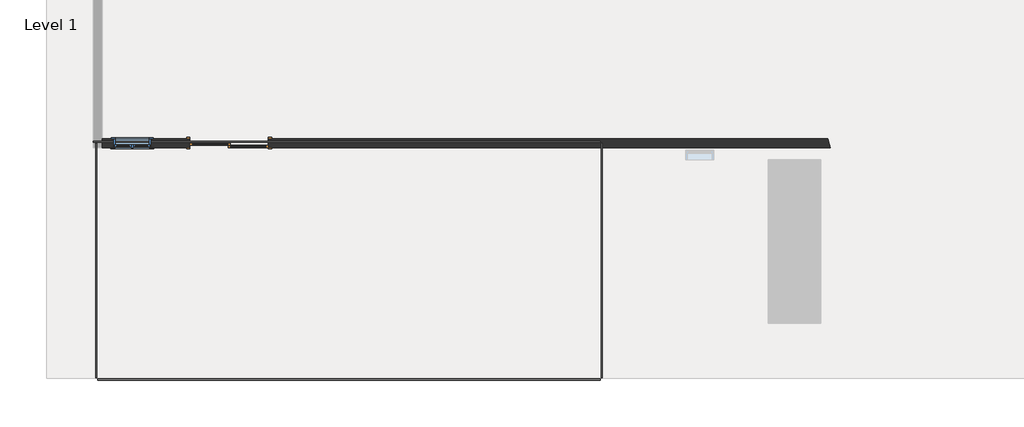
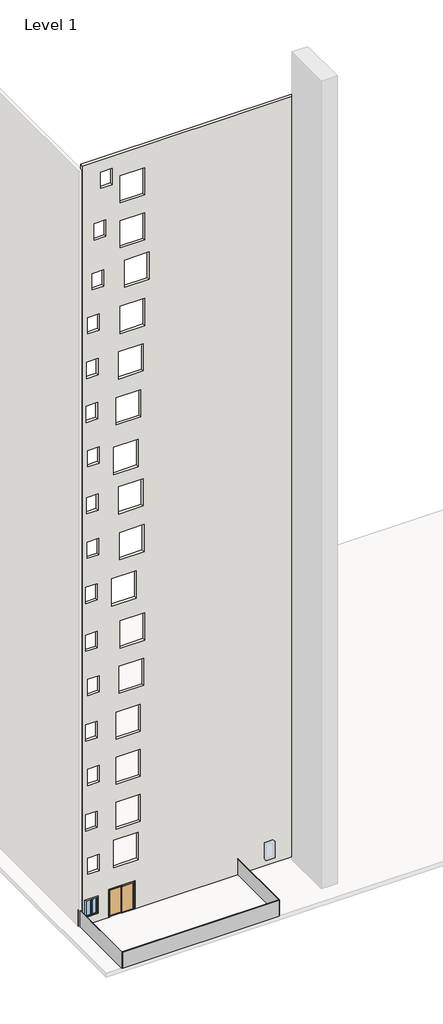
# One storey, part 1 of 3: 4 plates, 1 door, 1 wall, 1 window.
"""IFC4 building model written with IfcOpenShell, lengths in millimetres."""

from ifc_helpers import new_model, si_unit, frame, origin, place, context, project, spatial, polyline, circle_curve, transform, mapped, element, save
from ifc_brep_helpers import plane_surface, revolved_surface, advanced_brep
from components import door_076b30e0, system_panel_glazed_d9738348, system_panel_glazed_605ab5bb, system_panel_glazed_d159b752, window_bb17773d

model = new_model("IFC4")

# Units and contexts
model_context = context("Model", 3, world=origin())
ifc_project = project(units=[si_unit("LENGTHUNIT", "METRE", prefix="MILLI")], contexts=[model_context])

# Site, building, storey
site = spatial("IfcSite", under=ifc_project)
building = spatial("IfcBuilding", under=site)
storey = spatial("IfcBuildingStorey", under=building, Name="Level 1", Elevation=0.0)

# Door
placement = place(None, origin())
door_shape = door_076b30e0(model_context)
element("IfcDoor", 1, ObjectType="Door-Double-Sliding : 68\" x 80\"", at=placement, inside=storey, context=model_context, shape_type="MappedRepresentation", body=[
    mapped(door_shape, transform((-16826.585279, -12227.7237084, 0.0), x_axis=(-1.0, 0.0, 0.0), y_axis=(0.0, -1.0, 0.0), z_axis=(0.0, 0.0, 1.0))),
])

# Plates
system_panel_glazed_shape = system_panel_glazed_d9738348(model_context)
element("IfcPlate", 2, ObjectType="System Panel : Glazed", at=placement, inside=storey, context=model_context, shape_type="MappedRepresentation", body=[
    mapped(system_panel_glazed_shape, transform((-14188.160279, -17528.1341134, 0.0), x_axis=(-1.0, 0.0, 0.0), y_axis=(0.0, -1.0, 0.0), z_axis=(0.0, 0.0, 1.0))),
])
system_panel_glazed_2_shape = system_panel_glazed_605ab5bb(model_context)
element("IfcPlate", 3, ObjectType="System Panel : Glazed", at=placement, inside=storey, context=model_context, shape_type="MappedRepresentation", body=[
    mapped(system_panel_glazed_2_shape, transform((-19722.185279, -14941.4289109, 0.0), x_axis=(0.0, 1.0, 0.0), y_axis=(-1.0, 0.0, 0.0), z_axis=(0.0, 0.0, 1.0))),
])
element("IfcPlate", 4, ObjectType="System Panel : Glazed", at=placement, inside=storey, context=model_context, shape_type="MappedRepresentation", body=[
    mapped(system_panel_glazed_2_shape, transform((-8654.135279, -14941.4289109, 0.0), x_axis=(0.0, -1.0, 0.0), y_axis=(1.0, 0.0, 0.0), z_axis=(0.0, 0.0, 1.0))),
])
system_panel_glazed_3_shape = system_panel_glazed_d159b752(model_context)
element("IfcPlate", 5, ObjectType="System Panel : Glazed", at=placement, inside=storey, context=model_context, shape_type="MappedRepresentation", body=[
    mapped(system_panel_glazed_3_shape, transform((-14238.960279, -12354.7237084, 0.0), x_axis=(1.0, 0.0, 0.0), y_axis=(0.0, 1.0, 0.0), z_axis=(0.0, 0.0, 1.0))),
])

# Wall
element("IfcWall", 6, ObjectType="Generic - 8\"", at=placement, inside=storey, context=model_context, shape_type="AdvancedBrep", body=[
    advanced_brep(
    [(-17690.185279, -12253.1237084, 2032.0), (-17690.185279, -12253.1237084, 0.0), (-19620.585279, -12253.1237084, 0.0), (-19620.585279, -12253.1237084, 56730.1367162), (-3637.9363527, -12253.1237084, 56730.1367162), (-3637.9363527, -12253.1237084, 0.0), (-15962.985279, -12253.1237084, 0.0), (-15962.985279, -12253.1237084, 2032.0), (-18299.785279, -12253.1237084, 55822.814928), (-18299.785279, -12253.1237084, 54603.614928), (-17486.985279, -12253.1237084, 54603.614928), (-17486.985279, -12253.1237084, 55822.814928), (-18756.985279, -12253.1237084, 52120.8), (-18756.985279, -12253.1237084, 50901.6), (-17944.185279, -12253.1237084, 50901.6), (-17944.185279, -12253.1237084, 52120.8), (-18909.385279, -12253.1237084, 48463.2), (-18909.385279, -12253.1237084, 47244.0), (-18096.585279, -12253.1237084, 47244.0), (-18096.585279, -12253.1237084, 48463.2), (-19214.185279, -12253.1237084, 45287.1858782), (-19214.185279, -12253.1237084, 44067.9858782), (-18401.385279, -12253.1237084, 44067.9858782), (-18401.385279, -12253.1237084, 45287.1858782), (-19315.785279, -12253.1237084, 41987.2293246), (-19315.785279, -12253.1237084, 40768.0293246), (-18502.985279, -12253.1237084, 40768.0293246), (-18502.985279, -12253.1237084, 41987.2293246), (-19341.185279, -12253.1237084, 38709.6), (-19341.185279, -12253.1237084, 37490.4), (-18528.385279, -12253.1237084, 37490.4), (-18528.385279, -12253.1237084, 38709.6), (-19214.185279, -12253.1237084, 35356.8), (-19214.185279, -12253.1237084, 34137.6), (-18401.385279, -12253.1237084, 34137.6), (-18401.385279, -12253.1237084, 35356.8), (-19315.785279, -12253.1237084, 31888.4931655), (-19315.785279, -12253.1237084, 30669.2931655), (-18502.985279, -12253.1237084, 30669.2931655), (-18502.985279, -12253.1237084, 31888.4931655), (-19264.985279, -12253.1237084, 28544.0955009), (-19264.985279, -12253.1237084, 27324.8955009), (-18452.185279, -12253.1237084, 27324.8955009), (-18452.185279, -12253.1237084, 28544.0955009), (-19366.585279, -12253.1237084, 25208.6161382), (-19366.585279, -12253.1237084, 23989.4161382), (-18553.785279, -12253.1237084, 23989.4161382), (-18553.785279, -12253.1237084, 25208.6161382), (-19366.585279, -12253.1237084, 21640.8), (-19366.585279, -12253.1237084, 20421.6), (-18553.785279, -12253.1237084, 20421.6), (-18553.785279, -12253.1237084, 21640.8), (-19214.185279, -12253.1237084, 18288.0), (-19214.185279, -12253.1237084, 17068.8), (-18401.385279, -12253.1237084, 17068.8), (-18401.385279, -12253.1237084, 18288.0), (-19366.585279, -12253.1237084, 14935.2), (-19366.585279, -12253.1237084, 13716.0), (-18553.785279, -12253.1237084, 13716.0), (-18553.785279, -12253.1237084, 14935.2), (-19214.185279, -12253.1237084, 11582.4), (-19214.185279, -12253.1237084, 10363.2), (-18401.385279, -12253.1237084, 10363.2), (-18401.385279, -12253.1237084, 11582.4), (-19366.585279, -12253.1237084, 8229.6), (-19366.585279, -12253.1237084, 7010.4), (-18553.785279, -12253.1237084, 7010.4), (-18553.785279, -12253.1237084, 8229.6), (-19214.185279, -12253.1237084, 4949.2094119), (-19214.185279, -12253.1237084, 3730.0094119), (-18401.385279, -12253.1237084, 3730.0094119), (-18401.385279, -12253.1237084, 4949.2094119), (-19366.585279, -12253.1237084, 1819.2734472), (-19366.585279, -12253.1237084, 600.0734472), (-18553.785279, -12253.1237084, 600.0734472), (-18553.785279, -12253.1237084, 1819.2734472), (-15277.185279, -12253.1237084, 18491.2), (-17004.385279, -12253.1237084, 18491.2), (-17004.385279, -12253.1237084, 16459.2), (-15277.185279, -12253.1237084, 16459.2), (-15200.985279, -12253.1237084, 21844.0), (-16928.185279, -12253.1237084, 21844.0), (-16928.185279, -12253.1237084, 19812.0), (-15200.985279, -12253.1237084, 19812.0), (-15505.785279, -12253.1237084, 15138.4), (-17232.985279, -12253.1237084, 15138.4), (-17232.985279, -12253.1237084, 13106.4), (-15505.785279, -12253.1237084, 13106.4), (-15505.785279, -12253.1237084, 11785.6), (-17232.985279, -12253.1237084, 11785.6), (-17232.985279, -12253.1237084, 9753.6), (-15505.785279, -12253.1237084, 9753.6), (-15505.785279, -12253.1237084, 8432.8), (-17232.985279, -12253.1237084, 8432.8), (-17232.985279, -12253.1237084, 6400.8), (-15505.785279, -12253.1237084, 6400.8), (-15658.185279, -12253.1237084, 5624.1911771), (-17385.385279, -12253.1237084, 5624.1911771), (-17385.385279, -12253.1237084, 3592.1911771), (-15658.185279, -12253.1237084, 3592.1911771), (-15810.585279, -12253.1237084, 25196.8), (-17537.785279, -12253.1237084, 25196.8), (-17537.785279, -12253.1237084, 23164.8), (-15810.585279, -12253.1237084, 23164.8), (-15251.785279, -12253.1237084, 28462.5574534), (-16978.985279, -12253.1237084, 28462.5574534), (-16978.985279, -12253.1237084, 26430.5574534), (-15251.785279, -12253.1237084, 26430.5574534), (-15327.985279, -12253.1237084, 31902.4), (-17055.185279, -12253.1237084, 31902.4), (-17055.185279, -12253.1237084, 29870.4), (-15327.985279, -12253.1237084, 29870.4), (-15658.185279, -12253.1237084, 34950.4), (-17385.385279, -12253.1237084, 34950.4), (-17385.385279, -12253.1237084, 32918.4), (-15658.185279, -12253.1237084, 32918.4), (-15480.385279, -12253.1237084, 38608.0), (-17207.585279, -12253.1237084, 38608.0), (-17207.585279, -12253.1237084, 36576.0), (-15480.385279, -12253.1237084, 36576.0), (-15302.585279, -12253.1237084, 41960.8), (-17029.785279, -12253.1237084, 41960.8), (-17029.785279, -12253.1237084, 39928.8), (-15302.585279, -12253.1237084, 39928.8), (-15200.985279, -12253.1237084, 45313.6), (-16928.185279, -12253.1237084, 45313.6), (-16928.185279, -12253.1237084, 43281.6), (-15200.985279, -12253.1237084, 43281.6), (-14896.185279, -12253.1237084, 48666.4), (-16623.385279, -12253.1237084, 48666.4), (-16623.385279, -12253.1237084, 46634.4), (-14896.185279, -12253.1237084, 46634.4), (-15200.985279, -12253.1237084, 51714.4), (-16928.185279, -12253.1237084, 51714.4), (-16928.185279, -12253.1237084, 49682.4), (-15200.985279, -12253.1237084, 49682.4), (-15200.985279, -12253.1237084, 55067.2), (-16928.185279, -12253.1237084, 55067.2), (-16928.185279, -12253.1237084, 53035.2), (-15200.985279, -12253.1237084, 53035.2), (-19620.585279, -12456.3237084, 0.0), (-17690.185279, -12456.3237084, 0.0), (-17690.185279, -12456.3237084, 2032.0), (-15962.985279, -12456.3237084, 2032.0), (-15962.985279, -12456.3237084, 0.0), (-3801.1300045, -12456.3237084, 0.0), (-3592.0543777, -12456.3237084, 0.0), (-3592.0543777, -12456.3237084, 56730.1367162), (-3801.1300045, -12456.3237084, 56730.1367162), (-19620.585279, -12456.3237084, 56730.1367162), (-19620.585279, -12456.3237084, 56425.3367162), (-18299.785279, -12456.3237084, 55822.814928), (-17486.985279, -12456.3237084, 55822.814928), (-17486.985279, -12456.3237084, 54603.614928), (-18299.785279, -12456.3237084, 54603.614928), (-18756.985279, -12456.3237084, 52120.8), (-17944.185279, -12456.3237084, 52120.8), (-17944.185279, -12456.3237084, 50901.6), (-18756.985279, -12456.3237084, 50901.6), (-18909.385279, -12456.3237084, 48463.2), (-18096.585279, -12456.3237084, 48463.2), (-18096.585279, -12456.3237084, 47244.0), (-18909.385279, -12456.3237084, 47244.0), (-19214.185279, -12456.3237084, 45287.1858782), (-18401.385279, -12456.3237084, 45287.1858782), (-18401.385279, -12456.3237084, 44067.9858782), (-19214.185279, -12456.3237084, 44067.9858782), (-19315.785279, -12456.3237084, 41987.2293246), (-18502.985279, -12456.3237084, 41987.2293246), (-18502.985279, -12456.3237084, 40768.0293246), (-19315.785279, -12456.3237084, 40768.0293246), (-19341.185279, -12456.3237084, 38709.6), (-18528.385279, -12456.3237084, 38709.6), (-18528.385279, -12456.3237084, 37490.4), (-19341.185279, -12456.3237084, 37490.4), (-19214.185279, -12456.3237084, 35356.8), (-18401.385279, -12456.3237084, 35356.8), (-18401.385279, -12456.3237084, 34137.6), (-19214.185279, -12456.3237084, 34137.6), (-19315.785279, -12456.3237084, 31888.4931655), (-18502.985279, -12456.3237084, 31888.4931655), (-18502.985279, -12456.3237084, 30669.2931655), (-19315.785279, -12456.3237084, 30669.2931655), (-19264.985279, -12456.3237084, 28544.0955009), (-18452.185279, -12456.3237084, 28544.0955009), (-18452.185279, -12456.3237084, 27324.8955009), (-19264.985279, -12456.3237084, 27324.8955009), (-19366.585279, -12456.3237084, 25208.6161382), (-18553.785279, -12456.3237084, 25208.6161382), (-18553.785279, -12456.3237084, 23989.4161382), (-19366.585279, -12456.3237084, 23989.4161382), (-19366.585279, -12456.3237084, 21640.8), (-18553.785279, -12456.3237084, 21640.8), (-18553.785279, -12456.3237084, 20421.6), (-19366.585279, -12456.3237084, 20421.6), (-19214.185279, -12456.3237084, 18288.0), (-18401.385279, -12456.3237084, 18288.0), (-18401.385279, -12456.3237084, 17068.8), (-19214.185279, -12456.3237084, 17068.8), (-19366.585279, -12456.3237084, 14935.2), (-18553.785279, -12456.3237084, 14935.2), (-18553.785279, -12456.3237084, 13716.0), (-19366.585279, -12456.3237084, 13716.0), (-19214.185279, -12456.3237084, 11582.4), (-18401.385279, -12456.3237084, 11582.4), (-18401.385279, -12456.3237084, 10363.2), (-19214.185279, -12456.3237084, 10363.2), (-19366.585279, -12456.3237084, 8229.6), (-18553.785279, -12456.3237084, 8229.6), (-18553.785279, -12456.3237084, 7010.4), (-19366.585279, -12456.3237084, 7010.4), (-19214.185279, -12456.3237084, 4949.2094119), (-18401.385279, -12456.3237084, 4949.2094119), (-18401.385279, -12456.3237084, 3730.0094119), (-19214.185279, -12456.3237084, 3730.0094119), (-19366.585279, -12456.3237084, 1819.2734472), (-18553.785279, -12456.3237084, 1819.2734472), (-18553.785279, -12456.3237084, 600.0734472), (-19366.585279, -12456.3237084, 600.0734472), (-15277.185279, -12456.3237084, 18491.2), (-15277.185279, -12456.3237084, 16459.2), (-17004.385279, -12456.3237084, 16459.2), (-17004.385279, -12456.3237084, 18491.2), (-15200.985279, -12456.3237084, 21844.0), (-15200.985279, -12456.3237084, 19812.0), (-16928.185279, -12456.3237084, 19812.0), (-16928.185279, -12456.3237084, 21844.0), (-15505.785279, -12456.3237084, 15138.4), (-15505.785279, -12456.3237084, 13106.4), (-17232.985279, -12456.3237084, 13106.4), (-17232.985279, -12456.3237084, 15138.4), (-15505.785279, -12456.3237084, 11785.6), (-15505.785279, -12456.3237084, 9753.6), (-17232.985279, -12456.3237084, 9753.6), (-17232.985279, -12456.3237084, 11785.6), (-15505.785279, -12456.3237084, 8432.8), (-15505.785279, -12456.3237084, 6400.8), (-17232.985279, -12456.3237084, 6400.8), (-17232.985279, -12456.3237084, 8432.8), (-15658.185279, -12456.3237084, 5624.1911771), (-15658.185279, -12456.3237084, 3592.1911771), (-17385.385279, -12456.3237084, 3592.1911771), (-17385.385279, -12456.3237084, 5624.1911771), (-15810.585279, -12456.3237084, 25196.8), (-15810.585279, -12456.3237084, 23164.8), (-17537.785279, -12456.3237084, 23164.8), (-17537.785279, -12456.3237084, 25196.8), (-15251.785279, -12456.3237084, 28462.5574534), (-15251.785279, -12456.3237084, 26430.5574534), (-16978.985279, -12456.3237084, 26430.5574534), (-16978.985279, -12456.3237084, 28462.5574534), (-15327.985279, -12456.3237084, 31902.4), (-15327.985279, -12456.3237084, 29870.4), (-17055.185279, -12456.3237084, 29870.4), (-17055.185279, -12456.3237084, 31902.4), (-15658.185279, -12456.3237084, 34950.4), (-15658.185279, -12456.3237084, 32918.4), (-17385.385279, -12456.3237084, 32918.4), (-17385.385279, -12456.3237084, 34950.4), (-15480.385279, -12456.3237084, 38608.0), (-15480.385279, -12456.3237084, 36576.0), (-17207.585279, -12456.3237084, 36576.0), (-17207.585279, -12456.3237084, 38608.0), (-15302.585279, -12456.3237084, 41960.8), (-15302.585279, -12456.3237084, 39928.8), (-17029.785279, -12456.3237084, 39928.8), (-17029.785279, -12456.3237084, 41960.8), (-15200.985279, -12456.3237084, 45313.6), (-15200.985279, -12456.3237084, 43281.6), (-16928.185279, -12456.3237084, 43281.6), (-16928.185279, -12456.3237084, 45313.6), (-14896.185279, -12456.3237084, 48666.4), (-14896.185279, -12456.3237084, 46634.4), (-16623.385279, -12456.3237084, 46634.4), (-16623.385279, -12456.3237084, 48666.4), (-15200.985279, -12456.3237084, 51714.4), (-15200.985279, -12456.3237084, 49682.4), (-16928.185279, -12456.3237084, 49682.4), (-16928.185279, -12456.3237084, 51714.4), (-15200.985279, -12456.3237084, 55067.2), (-15200.985279, -12456.3237084, 53035.2), (-16928.185279, -12456.3237084, 53035.2), (-16928.185279, -12456.3237084, 55067.2)],
    [
        (0, 1),
        (1, 2),
        (2, 3),
        (3, 4),
        (4, 5),
        (5, 6),
        (6, 7),
        (7, 0),
        (8, 9),
        (9, 10),
        (10, 11),
        (11, 8),
        (12, 13),
        (13, 14),
        (14, 15),
        (15, 12),
        (16, 17),
        (17, 18),
        (18, 19),
        (19, 16),
        (20, 21),
        (21, 22),
        (22, 23),
        (23, 20),
        (24, 25),
        (25, 26),
        (26, 27),
        (27, 24),
        (28, 29),
        (29, 30),
        (30, 31),
        (31, 28),
        (32, 33),
        (33, 34),
        (34, 35),
        (35, 32),
        (36, 37),
        (37, 38),
        (38, 39),
        (39, 36),
        (40, 41),
        (41, 42),
        (42, 43),
        (43, 40),
        (44, 45),
        (45, 46),
        (46, 47),
        (47, 44),
        (48, 49),
        (49, 50),
        (50, 51),
        (51, 48),
        (52, 53),
        (53, 54),
        (54, 55),
        (55, 52),
        (56, 57),
        (57, 58),
        (58, 59),
        (59, 56),
        (60, 61),
        (61, 62),
        (62, 63),
        (63, 60),
        (64, 65),
        (65, 66),
        (66, 67),
        (67, 64),
        (68, 69),
        (69, 70),
        (70, 71),
        (71, 68),
        (72, 73),
        (73, 74),
        (74, 75),
        (75, 72),
        (76, 77),
        (77, 78),
        (78, 79),
        (79, 76),
        (80, 81),
        (81, 82),
        (82, 83),
        (83, 80),
        (84, 85),
        (85, 86),
        (86, 87),
        (87, 84),
        (88, 89),
        (89, 90),
        (90, 91),
        (91, 88),
        (92, 93),
        (93, 94),
        (94, 95),
        (95, 92),
        (96, 97),
        (97, 98),
        (98, 99),
        (99, 96),
        (100, 101),
        (101, 102),
        (102, 103),
        (103, 100),
        (104, 105),
        (105, 106),
        (106, 107),
        (107, 104),
        (108, 109),
        (109, 110),
        (110, 111),
        (111, 108),
        (112, 113),
        (113, 114),
        (114, 115),
        (115, 112),
        (116, 117),
        (117, 118),
        (118, 119),
        (119, 116),
        (120, 121),
        (121, 122),
        (122, 123),
        (123, 120),
        (124, 125),
        (125, 126),
        (126, 127),
        (127, 124),
        (128, 129),
        (129, 130),
        (130, 131),
        (131, 128),
        (132, 133),
        (133, 134),
        (134, 135),
        (135, 132),
        (136, 137),
        (137, 138),
        (138, 139),
        (139, 136),
        (140, 141),
        (141, 142),
        (142, 143),
        (143, 144),
        (144, 145),
        (145, 146),
        (146, 147),
        (147, 148),
        (148, 149),
        (149, 150),
        (150, 140),
        (151, 152),
        (152, 153),
        (153, 154),
        (154, 151),
        (155, 156),
        (156, 157),
        (157, 158),
        (158, 155),
        (159, 160),
        (160, 161),
        (161, 162),
        (162, 159),
        (163, 164),
        (164, 165),
        (165, 166),
        (166, 163),
        (167, 168),
        (168, 169),
        (169, 170),
        (170, 167),
        (171, 172),
        (172, 173),
        (173, 174),
        (174, 171),
        (175, 176),
        (176, 177),
        (177, 178),
        (178, 175),
        (179, 180),
        (180, 181),
        (181, 182),
        (182, 179),
        (183, 184),
        (184, 185),
        (185, 186),
        (186, 183),
        (187, 188),
        (188, 189),
        (189, 190),
        (190, 187),
        (191, 192),
        (192, 193),
        (193, 194),
        (194, 191),
        (195, 196),
        (196, 197),
        (197, 198),
        (198, 195),
        (199, 200),
        (200, 201),
        (201, 202),
        (202, 199),
        (203, 204),
        (204, 205),
        (205, 206),
        (206, 203),
        (207, 208),
        (208, 209),
        (209, 210),
        (210, 207),
        (211, 212),
        (212, 213),
        (213, 214),
        (214, 211),
        (215, 216),
        (216, 217),
        (217, 218),
        (218, 215),
        (219, 220),
        (220, 221),
        (221, 222),
        (222, 219),
        (223, 224),
        (224, 225),
        (225, 226),
        (226, 223),
        (227, 228),
        (228, 229),
        (229, 230),
        (230, 227),
        (231, 232),
        (232, 233),
        (233, 234),
        (234, 231),
        (235, 236),
        (236, 237),
        (237, 238),
        (238, 235),
        (239, 240),
        (240, 241),
        (241, 242),
        (242, 239),
        (243, 244),
        (244, 245),
        (245, 246),
        (246, 243),
        (247, 248),
        (248, 249),
        (249, 250),
        (250, 247),
        (251, 252),
        (252, 253),
        (253, 254),
        (254, 251),
        (255, 256),
        (256, 257),
        (257, 258),
        (258, 255),
        (259, 260),
        (260, 261),
        (261, 262),
        (262, 259),
        (263, 264),
        (264, 265),
        (265, 266),
        (266, 263),
        (267, 268),
        (268, 269),
        (269, 270),
        (270, 267),
        (271, 272),
        (272, 273),
        (273, 274),
        (274, 271),
        (275, 276),
        (276, 277),
        (277, 278),
        (278, 275),
        (279, 280),
        (280, 281),
        (281, 282),
        (282, 279),
        (5, 146, circle_curve(frame((1385.214721, -11225.6906671, 0.0), z_axis=(0.0, 0.0, 1.0), x_axis=(1.0, 0.0, 0.0)), 5127.1498284)),
        (144, 6),
        (1, 141),
        (140, 2),
        (3, 149),
        (147, 4, circle_curve(frame((1385.214721, -11225.6906671, 56730.1367162), z_axis=(0.0, 0.0, -1.0), x_axis=(1.0, 0.0, 0.0)), 5127.1498284)),
        (8, 151),
        (154, 9),
        (153, 10),
        (152, 11),
        (12, 155),
        (158, 13),
        (157, 14),
        (156, 15),
        (16, 159),
        (162, 17),
        (161, 18),
        (160, 19),
        (20, 163),
        (166, 21),
        (165, 22),
        (164, 23),
        (24, 167),
        (170, 25),
        (169, 26),
        (168, 27),
        (28, 171),
        (174, 29),
        (173, 30),
        (172, 31),
        (32, 175),
        (178, 33),
        (177, 34),
        (176, 35),
        (36, 179),
        (182, 37),
        (181, 38),
        (180, 39),
        (40, 183),
        (186, 41),
        (185, 42),
        (184, 43),
        (44, 187),
        (190, 45),
        (189, 46),
        (188, 47),
        (48, 191),
        (194, 49),
        (193, 50),
        (192, 51),
        (52, 195),
        (198, 53),
        (197, 54),
        (196, 55),
        (56, 199),
        (202, 57),
        (201, 58),
        (200, 59),
        (60, 203),
        (206, 61),
        (205, 62),
        (204, 63),
        (64, 207),
        (210, 65),
        (209, 66),
        (208, 67),
        (68, 211),
        (214, 69),
        (213, 70),
        (212, 71),
        (72, 215),
        (218, 73),
        (217, 74),
        (216, 75),
        (219, 76),
        (79, 220),
        (78, 221),
        (77, 222),
        (223, 80),
        (83, 224),
        (82, 225),
        (81, 226),
        (227, 84),
        (87, 228),
        (86, 229),
        (85, 230),
        (231, 88),
        (91, 232),
        (90, 233),
        (89, 234),
        (235, 92),
        (95, 236),
        (94, 237),
        (93, 238),
        (239, 96),
        (99, 240),
        (98, 241),
        (97, 242),
        (143, 7),
        (0, 142),
        (243, 100),
        (103, 244),
        (102, 245),
        (101, 246),
        (247, 104),
        (107, 248),
        (106, 249),
        (105, 250),
        (251, 108),
        (111, 252),
        (110, 253),
        (109, 254),
        (255, 112),
        (115, 256),
        (114, 257),
        (113, 258),
        (259, 116),
        (119, 260),
        (118, 261),
        (117, 262),
        (263, 120),
        (123, 264),
        (122, 265),
        (121, 266),
        (267, 124),
        (127, 268),
        (126, 269),
        (125, 270),
        (271, 128),
        (131, 272),
        (130, 273),
        (129, 274),
        (275, 132),
        (135, 276),
        (134, 277),
        (133, 278),
        (279, 136),
        (139, 280),
        (138, 281),
        (137, 282),
    ],
    [
        plane_surface(frame((25388.214721, -12253.1237084, 0.0), z_axis=(0.0, 1.0, 0.0), x_axis=(-1.0, 0.0, 0.0))),
        plane_surface(frame((25388.214721, -12456.3237084, 0.0), z_axis=(0.0, -1.0, 0.0), x_axis=(1.0, 0.0, 0.0))),
        plane_surface(frame((-3720.185279, -12253.1237084, 0.0), z_axis=(0.0, 0.0, -1.0), x_axis=(0.0, -1.0, 0.0))),
        plane_surface(frame((-19823.785279, -12253.1237084, 56730.1367162), z_axis=(0.0, 0.0, 1.0), x_axis=(0.0, -1.0, 0.0))),
        plane_surface(frame((-19620.585279, 12638.8762916, 0.0), z_axis=(-1.0, 0.0, 0.0), x_axis=(0.0, 1.0, 0.0))),
        revolved_surface(polyline([(6512.3645494, -11225.6906671, 0.0), (6512.3645494, -11225.6906671, 56730.1367162)]), (1385.214721, -11225.6906671, 0.0), (0.0, 0.0, -1.0)),
        plane_surface(frame((-18299.785279, -12253.1237084, 55822.814928), z_axis=(1.0, 0.0, 0.0), x_axis=(0.0, -1.0, 0.0))),
        plane_surface(frame((-18299.785279, -12253.1237084, 54603.614928), z_axis=(0.0, 0.0, 1.0), x_axis=(0.0, -1.0, 0.0))),
        plane_surface(frame((-17486.985279, -12253.1237084, 54603.614928), z_axis=(-1.0, 0.0, 0.0), x_axis=(0.0, -1.0, 0.0))),
        plane_surface(frame((-17486.985279, -12253.1237084, 55822.814928), z_axis=(0.0, 0.0, -1.0), x_axis=(0.0, -1.0, 0.0))),
        plane_surface(frame((-18756.985279, -12253.1237084, 52120.8), z_axis=(1.0, 0.0, 0.0), x_axis=(0.0, -1.0, 0.0))),
        plane_surface(frame((-18756.985279, -12253.1237084, 50901.6), z_axis=(0.0, 0.0, 1.0), x_axis=(0.0, -1.0, 0.0))),
        plane_surface(frame((-17944.185279, -12253.1237084, 50901.6), z_axis=(-1.0, 0.0, 0.0), x_axis=(0.0, -1.0, 0.0))),
        plane_surface(frame((-17944.185279, -12253.1237084, 52120.8), z_axis=(0.0, 0.0, -1.0), x_axis=(0.0, -1.0, 0.0))),
        plane_surface(frame((-18909.385279, -12253.1237084, 48463.2), z_axis=(1.0, 0.0, 0.0), x_axis=(0.0, -1.0, 0.0))),
        plane_surface(frame((-18909.385279, -12253.1237084, 47244.0), z_axis=(0.0, 0.0, 1.0), x_axis=(0.0, -1.0, 0.0))),
        plane_surface(frame((-18096.585279, -12253.1237084, 47244.0), z_axis=(-1.0, 0.0, 0.0), x_axis=(0.0, -1.0, 0.0))),
        plane_surface(frame((-18096.585279, -12253.1237084, 48463.2), z_axis=(0.0, 0.0, -1.0), x_axis=(0.0, -1.0, 0.0))),
        plane_surface(frame((-19214.185279, -12253.1237084, 45287.1858782), z_axis=(1.0, 0.0, 0.0), x_axis=(0.0, -1.0, 0.0))),
        plane_surface(frame((-19214.185279, -12253.1237084, 44067.9858782), z_axis=(0.0, 0.0, 1.0), x_axis=(0.0, -1.0, 0.0))),
        plane_surface(frame((-18401.385279, -12253.1237084, 44067.9858782), z_axis=(-1.0, 0.0, 0.0), x_axis=(0.0, -1.0, 0.0))),
        plane_surface(frame((-18401.385279, -12253.1237084, 45287.1858782), z_axis=(0.0, 0.0, -1.0), x_axis=(0.0, -1.0, 0.0))),
        plane_surface(frame((-19315.785279, -12253.1237084, 41987.2293246), z_axis=(1.0, 0.0, 0.0), x_axis=(0.0, -1.0, 0.0))),
        plane_surface(frame((-19315.785279, -12253.1237084, 40768.0293246), z_axis=(0.0, 0.0, 1.0), x_axis=(0.0, -1.0, 0.0))),
        plane_surface(frame((-18502.985279, -12253.1237084, 40768.0293246), z_axis=(-1.0, 0.0, 0.0), x_axis=(0.0, -1.0, 0.0))),
        plane_surface(frame((-18502.985279, -12253.1237084, 41987.2293246), z_axis=(0.0, 0.0, -1.0), x_axis=(0.0, -1.0, 0.0))),
        plane_surface(frame((-19341.185279, -12253.1237084, 38709.6), z_axis=(1.0, 0.0, 0.0), x_axis=(0.0, -1.0, 0.0))),
        plane_surface(frame((-19341.185279, -12253.1237084, 37490.4), z_axis=(0.0, 0.0, 1.0), x_axis=(0.0, -1.0, 0.0))),
        plane_surface(frame((-18528.385279, -12253.1237084, 37490.4), z_axis=(-1.0, 0.0, 0.0), x_axis=(0.0, -1.0, 0.0))),
        plane_surface(frame((-18528.385279, -12253.1237084, 38709.6), z_axis=(0.0, 0.0, -1.0), x_axis=(0.0, -1.0, 0.0))),
        plane_surface(frame((-19214.185279, -12253.1237084, 35356.8), z_axis=(1.0, 0.0, 0.0), x_axis=(0.0, -1.0, 0.0))),
        plane_surface(frame((-19214.185279, -12253.1237084, 34137.6), z_axis=(0.0, 0.0, 1.0), x_axis=(0.0, -1.0, 0.0))),
        plane_surface(frame((-18401.385279, -12253.1237084, 34137.6), z_axis=(-1.0, 0.0, 0.0), x_axis=(0.0, -1.0, 0.0))),
        plane_surface(frame((-18401.385279, -12253.1237084, 35356.8), z_axis=(0.0, 0.0, -1.0), x_axis=(0.0, -1.0, 0.0))),
        plane_surface(frame((-19315.785279, -12253.1237084, 31888.4931655), z_axis=(1.0, 0.0, 0.0), x_axis=(0.0, -1.0, 0.0))),
        plane_surface(frame((-19315.785279, -12253.1237084, 30669.2931655), z_axis=(0.0, 0.0, 1.0), x_axis=(0.0, -1.0, 0.0))),
        plane_surface(frame((-18502.985279, -12253.1237084, 30669.2931655), z_axis=(-1.0, 0.0, 0.0), x_axis=(0.0, -1.0, 0.0))),
        plane_surface(frame((-18502.985279, -12253.1237084, 31888.4931655), z_axis=(0.0, 0.0, -1.0), x_axis=(0.0, -1.0, 0.0))),
        plane_surface(frame((-19264.985279, -12253.1237084, 28544.0955009), z_axis=(1.0, 0.0, 0.0), x_axis=(0.0, -1.0, 0.0))),
        plane_surface(frame((-19264.985279, -12253.1237084, 27324.8955009), z_axis=(0.0, 0.0, 1.0), x_axis=(0.0, -1.0, 0.0))),
        plane_surface(frame((-18452.185279, -12253.1237084, 27324.8955009), z_axis=(-1.0, 0.0, 0.0), x_axis=(0.0, -1.0, 0.0))),
        plane_surface(frame((-18452.185279, -12253.1237084, 28544.0955009), z_axis=(0.0, 0.0, -1.0), x_axis=(0.0, -1.0, 0.0))),
        plane_surface(frame((-19366.585279, -12253.1237084, 25208.6161382), z_axis=(1.0, 0.0, 0.0), x_axis=(0.0, -1.0, 0.0))),
        plane_surface(frame((-19366.585279, -12253.1237084, 23989.4161382), z_axis=(0.0, 0.0, 1.0), x_axis=(0.0, -1.0, 0.0))),
        plane_surface(frame((-18553.785279, -12253.1237084, 23989.4161382), z_axis=(-1.0, 0.0, 0.0), x_axis=(0.0, -1.0, 0.0))),
        plane_surface(frame((-18553.785279, -12253.1237084, 25208.6161382), z_axis=(0.0, 0.0, -1.0), x_axis=(0.0, -1.0, 0.0))),
        plane_surface(frame((-19366.585279, -12253.1237084, 21640.8), z_axis=(1.0, 0.0, 0.0), x_axis=(0.0, -1.0, 0.0))),
        plane_surface(frame((-19366.585279, -12253.1237084, 20421.6), z_axis=(0.0, 0.0, 1.0), x_axis=(0.0, -1.0, 0.0))),
        plane_surface(frame((-18553.785279, -12253.1237084, 20421.6), z_axis=(-1.0, 0.0, 0.0), x_axis=(0.0, -1.0, 0.0))),
        plane_surface(frame((-18553.785279, -12253.1237084, 21640.8), z_axis=(0.0, 0.0, -1.0), x_axis=(0.0, -1.0, 0.0))),
        plane_surface(frame((-19214.185279, -12253.1237084, 18288.0), z_axis=(1.0, 0.0, 0.0), x_axis=(0.0, -1.0, 0.0))),
        plane_surface(frame((-19214.185279, -12253.1237084, 17068.8), z_axis=(0.0, 0.0, 1.0), x_axis=(0.0, -1.0, 0.0))),
        plane_surface(frame((-18401.385279, -12253.1237084, 17068.8), z_axis=(-1.0, 0.0, 0.0), x_axis=(0.0, -1.0, 0.0))),
        plane_surface(frame((-18401.385279, -12253.1237084, 18288.0), z_axis=(0.0, 0.0, -1.0), x_axis=(0.0, -1.0, 0.0))),
        plane_surface(frame((-19366.585279, -12253.1237084, 14935.2), z_axis=(1.0, 0.0, 0.0), x_axis=(0.0, -1.0, 0.0))),
        plane_surface(frame((-19366.585279, -12253.1237084, 13716.0), z_axis=(0.0, 0.0, 1.0), x_axis=(0.0, -1.0, 0.0))),
        plane_surface(frame((-18553.785279, -12253.1237084, 13716.0), z_axis=(-1.0, 0.0, 0.0), x_axis=(0.0, -1.0, 0.0))),
        plane_surface(frame((-18553.785279, -12253.1237084, 14935.2), z_axis=(0.0, 0.0, -1.0), x_axis=(0.0, -1.0, 0.0))),
        plane_surface(frame((-19214.185279, -12253.1237084, 11582.4), z_axis=(1.0, 0.0, 0.0), x_axis=(0.0, -1.0, 0.0))),
        plane_surface(frame((-19214.185279, -12253.1237084, 10363.2), z_axis=(0.0, 0.0, 1.0), x_axis=(0.0, -1.0, 0.0))),
        plane_surface(frame((-18401.385279, -12253.1237084, 10363.2), z_axis=(-1.0, 0.0, 0.0), x_axis=(0.0, -1.0, 0.0))),
        plane_surface(frame((-18401.385279, -12253.1237084, 11582.4), z_axis=(0.0, 0.0, -1.0), x_axis=(0.0, -1.0, 0.0))),
        plane_surface(frame((-19366.585279, -12253.1237084, 8229.6), z_axis=(1.0, 0.0, 0.0), x_axis=(0.0, -1.0, 0.0))),
        plane_surface(frame((-19366.585279, -12253.1237084, 7010.4), z_axis=(0.0, 0.0, 1.0), x_axis=(0.0, -1.0, 0.0))),
        plane_surface(frame((-18553.785279, -12253.1237084, 7010.4), z_axis=(-1.0, 0.0, 0.0), x_axis=(0.0, -1.0, 0.0))),
        plane_surface(frame((-18553.785279, -12253.1237084, 8229.6), z_axis=(0.0, 0.0, -1.0), x_axis=(0.0, -1.0, 0.0))),
        plane_surface(frame((-19214.185279, -12253.1237084, 4949.2094119), z_axis=(1.0, 0.0, 0.0), x_axis=(0.0, -1.0, 0.0))),
        plane_surface(frame((-19214.185279, -12253.1237084, 3730.0094119), z_axis=(0.0, 0.0, 1.0), x_axis=(0.0, -1.0, 0.0))),
        plane_surface(frame((-18401.385279, -12253.1237084, 3730.0094119), z_axis=(-1.0, 0.0, 0.0), x_axis=(0.0, -1.0, 0.0))),
        plane_surface(frame((-18401.385279, -12253.1237084, 4949.2094119), z_axis=(0.0, 0.0, -1.0), x_axis=(0.0, -1.0, 0.0))),
        plane_surface(frame((-19366.585279, -12253.1237084, 1819.2734472), z_axis=(1.0, 0.0, 0.0), x_axis=(0.0, -1.0, 0.0))),
        plane_surface(frame((-19366.585279, -12253.1237084, 600.0734472), z_axis=(0.0, 0.0, 1.0), x_axis=(0.0, -1.0, 0.0))),
        plane_surface(frame((-18553.785279, -12253.1237084, 600.0734472), z_axis=(-1.0, 0.0, 0.0), x_axis=(0.0, -1.0, 0.0))),
        plane_surface(frame((-18553.785279, -12253.1237084, 1819.2734472), z_axis=(0.0, 0.0, -1.0), x_axis=(0.0, -1.0, 0.0))),
        plane_surface(frame((-15277.185279, -12456.3237084, 18491.2), z_axis=(-1.0, 0.0, 0.0), x_axis=(0.0, 1.0, 0.0))),
        plane_surface(frame((-15277.185279, -12456.3237084, 16459.2), z_axis=(0.0, 0.0, 1.0), x_axis=(0.0, 1.0, 0.0))),
        plane_surface(frame((-17004.385279, -12456.3237084, 16459.2), z_axis=(1.0, 0.0, 0.0), x_axis=(0.0, 1.0, 0.0))),
        plane_surface(frame((-17004.385279, -12456.3237084, 18491.2), z_axis=(0.0, 0.0, -1.0), x_axis=(0.0, 1.0, 0.0))),
        plane_surface(frame((-15200.985279, -12456.3237084, 21844.0), z_axis=(-1.0, 0.0, 0.0), x_axis=(0.0, 1.0, 0.0))),
        plane_surface(frame((-15200.985279, -12456.3237084, 19812.0), z_axis=(0.0, 0.0, 1.0), x_axis=(0.0, 1.0, 0.0))),
        plane_surface(frame((-16928.185279, -12456.3237084, 19812.0), z_axis=(1.0, 0.0, 0.0), x_axis=(0.0, 1.0, 0.0))),
        plane_surface(frame((-16928.185279, -12456.3237084, 21844.0), z_axis=(0.0, 0.0, -1.0), x_axis=(0.0, 1.0, 0.0))),
        plane_surface(frame((-15505.785279, -12456.3237084, 15138.4), z_axis=(-1.0, 0.0, 0.0), x_axis=(0.0, 1.0, 0.0))),
        plane_surface(frame((-15505.785279, -12456.3237084, 13106.4), z_axis=(0.0, 0.0, 1.0), x_axis=(0.0, 1.0, 0.0))),
        plane_surface(frame((-17232.985279, -12456.3237084, 13106.4), z_axis=(1.0, 0.0, 0.0), x_axis=(0.0, 1.0, 0.0))),
        plane_surface(frame((-17232.985279, -12456.3237084, 15138.4), z_axis=(0.0, 0.0, -1.0), x_axis=(0.0, 1.0, 0.0))),
        plane_surface(frame((-15505.785279, -12456.3237084, 11785.6), z_axis=(-1.0, 0.0, 0.0), x_axis=(0.0, 1.0, 0.0))),
        plane_surface(frame((-15505.785279, -12456.3237084, 9753.6), z_axis=(0.0, 0.0, 1.0), x_axis=(0.0, 1.0, 0.0))),
        plane_surface(frame((-17232.985279, -12456.3237084, 9753.6), z_axis=(1.0, 0.0, 0.0), x_axis=(0.0, 1.0, 0.0))),
        plane_surface(frame((-17232.985279, -12456.3237084, 11785.6), z_axis=(0.0, 0.0, -1.0), x_axis=(0.0, 1.0, 0.0))),
        plane_surface(frame((-15505.785279, -12456.3237084, 8432.8), z_axis=(-1.0, 0.0, 0.0), x_axis=(0.0, 1.0, 0.0))),
        plane_surface(frame((-15505.785279, -12456.3237084, 6400.8), z_axis=(0.0, 0.0, 1.0), x_axis=(0.0, 1.0, 0.0))),
        plane_surface(frame((-17232.985279, -12456.3237084, 6400.8), z_axis=(1.0, 0.0, 0.0), x_axis=(0.0, 1.0, 0.0))),
        plane_surface(frame((-17232.985279, -12456.3237084, 8432.8), z_axis=(0.0, 0.0, -1.0), x_axis=(0.0, 1.0, 0.0))),
        plane_surface(frame((-15658.185279, -12456.3237084, 5624.1911771), z_axis=(-1.0, 0.0, 0.0), x_axis=(0.0, 1.0, 0.0))),
        plane_surface(frame((-15658.185279, -12456.3237084, 3592.1911771), z_axis=(0.0, 0.0, 1.0), x_axis=(0.0, 1.0, 0.0))),
        plane_surface(frame((-17385.385279, -12456.3237084, 3592.1911771), z_axis=(1.0, 0.0, 0.0), x_axis=(0.0, 1.0, 0.0))),
        plane_surface(frame((-17385.385279, -12456.3237084, 5624.1911771), z_axis=(0.0, 0.0, -1.0), x_axis=(0.0, 1.0, 0.0))),
        plane_surface(frame((-15962.985279, -12456.3237084, 2032.0), z_axis=(-1.0, 0.0, 0.0), x_axis=(0.0, 1.0, 0.0))),
        plane_surface(frame((-17690.185279, -12456.3237084, 0.0), z_axis=(1.0, 0.0, 0.0), x_axis=(0.0, 1.0, 0.0))),
        plane_surface(frame((-17690.185279, -12456.3237084, 2032.0), z_axis=(0.0, 0.0, -1.0), x_axis=(0.0, 1.0, 0.0))),
        plane_surface(frame((-15810.585279, -12456.3237084, 25196.8), z_axis=(-1.0, 0.0, 0.0), x_axis=(0.0, 1.0, 0.0))),
        plane_surface(frame((-15810.585279, -12456.3237084, 23164.8), z_axis=(0.0, 0.0, 1.0), x_axis=(0.0, 1.0, 0.0))),
        plane_surface(frame((-17537.785279, -12456.3237084, 23164.8), z_axis=(1.0, 0.0, 0.0), x_axis=(0.0, 1.0, 0.0))),
        plane_surface(frame((-17537.785279, -12456.3237084, 25196.8), z_axis=(0.0, 0.0, -1.0), x_axis=(0.0, 1.0, 0.0))),
        plane_surface(frame((-15251.785279, -12456.3237084, 28462.5574534), z_axis=(-1.0, 0.0, 0.0), x_axis=(0.0, 1.0, 0.0))),
        plane_surface(frame((-15251.785279, -12456.3237084, 26430.5574534), z_axis=(0.0, 0.0, 1.0), x_axis=(0.0, 1.0, 0.0))),
        plane_surface(frame((-16978.985279, -12456.3237084, 26430.5574534), z_axis=(1.0, 0.0, 0.0), x_axis=(0.0, 1.0, 0.0))),
        plane_surface(frame((-16978.985279, -12456.3237084, 28462.5574534), z_axis=(0.0, 0.0, -1.0), x_axis=(0.0, 1.0, 0.0))),
        plane_surface(frame((-15327.985279, -12456.3237084, 31902.4), z_axis=(-1.0, 0.0, 0.0), x_axis=(0.0, 1.0, 0.0))),
        plane_surface(frame((-15327.985279, -12456.3237084, 29870.4), z_axis=(0.0, 0.0, 1.0), x_axis=(0.0, 1.0, 0.0))),
        plane_surface(frame((-17055.185279, -12456.3237084, 29870.4), z_axis=(1.0, 0.0, 0.0), x_axis=(0.0, 1.0, 0.0))),
        plane_surface(frame((-17055.185279, -12456.3237084, 31902.4), z_axis=(0.0, 0.0, -1.0), x_axis=(0.0, 1.0, 0.0))),
        plane_surface(frame((-15658.185279, -12456.3237084, 34950.4), z_axis=(-1.0, 0.0, 0.0), x_axis=(0.0, 1.0, 0.0))),
        plane_surface(frame((-15658.185279, -12456.3237084, 32918.4), z_axis=(0.0, 0.0, 1.0), x_axis=(0.0, 1.0, 0.0))),
        plane_surface(frame((-17385.385279, -12456.3237084, 32918.4), z_axis=(1.0, 0.0, 0.0), x_axis=(0.0, 1.0, 0.0))),
        plane_surface(frame((-17385.385279, -12456.3237084, 34950.4), z_axis=(0.0, 0.0, -1.0), x_axis=(0.0, 1.0, 0.0))),
        plane_surface(frame((-15480.385279, -12456.3237084, 38608.0), z_axis=(-1.0, 0.0, 0.0), x_axis=(0.0, 1.0, 0.0))),
        plane_surface(frame((-15480.385279, -12456.3237084, 36576.0), z_axis=(0.0, 0.0, 1.0), x_axis=(0.0, 1.0, 0.0))),
        plane_surface(frame((-17207.585279, -12456.3237084, 36576.0), z_axis=(1.0, 0.0, 0.0), x_axis=(0.0, 1.0, 0.0))),
        plane_surface(frame((-17207.585279, -12456.3237084, 38608.0), z_axis=(0.0, 0.0, -1.0), x_axis=(0.0, 1.0, 0.0))),
        plane_surface(frame((-15302.585279, -12456.3237084, 41960.8), z_axis=(-1.0, 0.0, 0.0), x_axis=(0.0, 1.0, 0.0))),
        plane_surface(frame((-15302.585279, -12456.3237084, 39928.8), z_axis=(0.0, 0.0, 1.0), x_axis=(0.0, 1.0, 0.0))),
        plane_surface(frame((-17029.785279, -12456.3237084, 39928.8), z_axis=(1.0, 0.0, 0.0), x_axis=(0.0, 1.0, 0.0))),
        plane_surface(frame((-17029.785279, -12456.3237084, 41960.8), z_axis=(0.0, 0.0, -1.0), x_axis=(0.0, 1.0, 0.0))),
        plane_surface(frame((-15200.985279, -12456.3237084, 45313.6), z_axis=(-1.0, 0.0, 0.0), x_axis=(0.0, 1.0, 0.0))),
        plane_surface(frame((-15200.985279, -12456.3237084, 43281.6), z_axis=(0.0, 0.0, 1.0), x_axis=(0.0, 1.0, 0.0))),
        plane_surface(frame((-16928.185279, -12456.3237084, 43281.6), z_axis=(1.0, 0.0, 0.0), x_axis=(0.0, 1.0, 0.0))),
        plane_surface(frame((-16928.185279, -12456.3237084, 45313.6), z_axis=(0.0, 0.0, -1.0), x_axis=(0.0, 1.0, 0.0))),
        plane_surface(frame((-14896.185279, -12456.3237084, 48666.4), z_axis=(-1.0, 0.0, 0.0), x_axis=(0.0, 1.0, 0.0))),
        plane_surface(frame((-14896.185279, -12456.3237084, 46634.4), z_axis=(0.0, 0.0, 1.0), x_axis=(0.0, 1.0, 0.0))),
        plane_surface(frame((-16623.385279, -12456.3237084, 46634.4), z_axis=(1.0, 0.0, 0.0), x_axis=(0.0, 1.0, 0.0))),
        plane_surface(frame((-16623.385279, -12456.3237084, 48666.4), z_axis=(0.0, 0.0, -1.0), x_axis=(0.0, 1.0, 0.0))),
        plane_surface(frame((-15200.985279, -12456.3237084, 51714.4), z_axis=(-1.0, 0.0, 0.0), x_axis=(0.0, 1.0, 0.0))),
        plane_surface(frame((-15200.985279, -12456.3237084, 49682.4), z_axis=(0.0, 0.0, 1.0), x_axis=(0.0, 1.0, 0.0))),
        plane_surface(frame((-16928.185279, -12456.3237084, 49682.4), z_axis=(1.0, 0.0, 0.0), x_axis=(0.0, 1.0, 0.0))),
        plane_surface(frame((-16928.185279, -12456.3237084, 51714.4), z_axis=(0.0, 0.0, -1.0), x_axis=(0.0, 1.0, 0.0))),
        plane_surface(frame((-15200.985279, -12456.3237084, 55067.2), z_axis=(-1.0, 0.0, 0.0), x_axis=(0.0, 1.0, 0.0))),
        plane_surface(frame((-15200.985279, -12456.3237084, 53035.2), z_axis=(0.0, 0.0, 1.0), x_axis=(0.0, 1.0, 0.0))),
        plane_surface(frame((-16928.185279, -12456.3237084, 53035.2), z_axis=(1.0, 0.0, 0.0), x_axis=(0.0, 1.0, 0.0))),
        plane_surface(frame((-16928.185279, -12456.3237084, 55067.2), z_axis=(0.0, 0.0, -1.0), x_axis=(0.0, 1.0, 0.0))),
    ],
    [
        (0, [[1, 2, 3, 4, 5, 6, 7, 8], [9, 10, 11, 12], [13, 14, 15, 16], [17, 18, 19, 20], [21, 22, 23, 24], [25, 26, 27, 28], [29, 30, 31, 32], [33, 34, 35, 36], [37, 38, 39, 40], [41, 42, 43, 44], [45, 46, 47, 48], [49, 50, 51, 52], [53, 54, 55, 56], [57, 58, 59, 60], [61, 62, 63, 64], [65, 66, 67, 68], [69, 70, 71, 72], [73, 74, 75, 76], [77, 78, 79, 80], [81, 82, 83, 84], [85, 86, 87, 88], [89, 90, 91, 92], [93, 94, 95, 96], [97, 98, 99, 100], [101, 102, 103, 104], [105, 106, 107, 108], [109, 110, 111, 112], [113, 114, 115, 116], [117, 118, 119, 120], [121, 122, 123, 124], [125, 126, 127, 128], [129, 130, 131, 132], [133, 134, 135, 136], [137, 138, 139, 140]]),
        (1, [[141, 142, 143, 144, 145, 146, 147, 148, 149, 150, 151], [152, 153, 154, 155], [156, 157, 158, 159], [160, 161, 162, 163], [164, 165, 166, 167], [168, 169, 170, 171], [172, 173, 174, 175], [176, 177, 178, 179], [180, 181, 182, 183], [184, 185, 186, 187], [188, 189, 190, 191], [192, 193, 194, 195], [196, 197, 198, 199], [200, 201, 202, 203], [204, 205, 206, 207], [208, 209, 210, 211], [212, 213, 214, 215], [216, 217, 218, 219], [220, 221, 222, 223], [224, 225, 226, 227], [228, 229, 230, 231], [232, 233, 234, 235], [236, 237, 238, 239], [240, 241, 242, 243], [244, 245, 246, 247], [248, 249, 250, 251], [252, 253, 254, 255], [256, 257, 258, 259], [260, 261, 262, 263], [264, 265, 266, 267], [268, 269, 270, 271], [272, 273, 274, 275], [276, 277, 278, 279], [280, 281, 282, 283]]),
        (2, [[-6, 284, -146, -145, 285]]),
        (2, [[-2, 286, -141, 287]]),
        (3, [[-4, 288, -149, -148, 289]]),
        (4, [[-3, -287, -151, -150, -288]]),
        (5, [[-5, -289, -147, -284]]),
        (6, [[-9, 290, -155, 291]]),
        (7, [[-10, -291, -154, 292]]),
        (8, [[-11, -292, -153, 293]]),
        (9, [[-12, -293, -152, -290]]),
        (10, [[-13, 294, -159, 295]]),
        (11, [[-14, -295, -158, 296]]),
        (12, [[-15, -296, -157, 297]]),
        (13, [[-16, -297, -156, -294]]),
        (14, [[-17, 298, -163, 299]]),
        (15, [[-18, -299, -162, 300]]),
        (16, [[-19, -300, -161, 301]]),
        (17, [[-20, -301, -160, -298]]),
        (18, [[-21, 302, -167, 303]]),
        (19, [[-22, -303, -166, 304]]),
        (20, [[-23, -304, -165, 305]]),
        (21, [[-24, -305, -164, -302]]),
        (22, [[-25, 306, -171, 307]]),
        (23, [[-26, -307, -170, 308]]),
        (24, [[-27, -308, -169, 309]]),
        (25, [[-28, -309, -168, -306]]),
        (26, [[-29, 310, -175, 311]]),
        (27, [[-30, -311, -174, 312]]),
        (28, [[-31, -312, -173, 313]]),
        (29, [[-32, -313, -172, -310]]),
        (30, [[-33, 314, -179, 315]]),
        (31, [[-34, -315, -178, 316]]),
        (32, [[-35, -316, -177, 317]]),
        (33, [[-36, -317, -176, -314]]),
        (34, [[-37, 318, -183, 319]]),
        (35, [[-38, -319, -182, 320]]),
        (36, [[-39, -320, -181, 321]]),
        (37, [[-40, -321, -180, -318]]),
        (38, [[-41, 322, -187, 323]]),
        (39, [[-42, -323, -186, 324]]),
        (40, [[-43, -324, -185, 325]]),
        (41, [[-44, -325, -184, -322]]),
        (42, [[-45, 326, -191, 327]]),
        (43, [[-46, -327, -190, 328]]),
        (44, [[-47, -328, -189, 329]]),
        (45, [[-48, -329, -188, -326]]),
        (46, [[-49, 330, -195, 331]]),
        (47, [[-50, -331, -194, 332]]),
        (48, [[-51, -332, -193, 333]]),
        (49, [[-52, -333, -192, -330]]),
        (50, [[-53, 334, -199, 335]]),
        (51, [[-54, -335, -198, 336]]),
        (52, [[-55, -336, -197, 337]]),
        (53, [[-56, -337, -196, -334]]),
        (54, [[-57, 338, -203, 339]]),
        (55, [[-58, -339, -202, 340]]),
        (56, [[-59, -340, -201, 341]]),
        (57, [[-60, -341, -200, -338]]),
        (58, [[-61, 342, -207, 343]]),
        (59, [[-62, -343, -206, 344]]),
        (60, [[-63, -344, -205, 345]]),
        (61, [[-64, -345, -204, -342]]),
        (62, [[-65, 346, -211, 347]]),
        (63, [[-66, -347, -210, 348]]),
        (64, [[-67, -348, -209, 349]]),
        (65, [[-68, -349, -208, -346]]),
        (66, [[-69, 350, -215, 351]]),
        (67, [[-70, -351, -214, 352]]),
        (68, [[-71, -352, -213, 353]]),
        (69, [[-72, -353, -212, -350]]),
        (70, [[-73, 354, -219, 355]]),
        (71, [[-74, -355, -218, 356]]),
        (72, [[-75, -356, -217, 357]]),
        (73, [[-76, -357, -216, -354]]),
        (74, [[-220, 358, -80, 359]]),
        (75, [[-221, -359, -79, 360]]),
        (76, [[-222, -360, -78, 361]]),
        (77, [[-223, -361, -77, -358]]),
        (78, [[-224, 362, -84, 363]]),
        (79, [[-225, -363, -83, 364]]),
        (80, [[-226, -364, -82, 365]]),
        (81, [[-227, -365, -81, -362]]),
        (82, [[-228, 366, -88, 367]]),
        (83, [[-229, -367, -87, 368]]),
        (84, [[-230, -368, -86, 369]]),
        (85, [[-231, -369, -85, -366]]),
        (86, [[-232, 370, -92, 371]]),
        (87, [[-233, -371, -91, 372]]),
        (88, [[-234, -372, -90, 373]]),
        (89, [[-235, -373, -89, -370]]),
        (90, [[-236, 374, -96, 375]]),
        (91, [[-237, -375, -95, 376]]),
        (92, [[-238, -376, -94, 377]]),
        (93, [[-239, -377, -93, -374]]),
        (94, [[-240, 378, -100, 379]]),
        (95, [[-241, -379, -99, 380]]),
        (96, [[-242, -380, -98, 381]]),
        (97, [[-243, -381, -97, -378]]),
        (98, [[-144, 382, -7, -285]]),
        (99, [[-142, -286, -1, 383]]),
        (100, [[-143, -383, -8, -382]]),
        (101, [[-244, 384, -104, 385]]),
        (102, [[-245, -385, -103, 386]]),
        (103, [[-246, -386, -102, 387]]),
        (104, [[-247, -387, -101, -384]]),
        (105, [[-248, 388, -108, 389]]),
        (106, [[-249, -389, -107, 390]]),
        (107, [[-250, -390, -106, 391]]),
        (108, [[-251, -391, -105, -388]]),
        (109, [[-252, 392, -112, 393]]),
        (110, [[-253, -393, -111, 394]]),
        (111, [[-254, -394, -110, 395]]),
        (112, [[-255, -395, -109, -392]]),
        (113, [[-256, 396, -116, 397]]),
        (114, [[-257, -397, -115, 398]]),
        (115, [[-258, -398, -114, 399]]),
        (116, [[-259, -399, -113, -396]]),
        (117, [[-260, 400, -120, 401]]),
        (118, [[-261, -401, -119, 402]]),
        (119, [[-262, -402, -118, 403]]),
        (120, [[-263, -403, -117, -400]]),
        (121, [[-264, 404, -124, 405]]),
        (122, [[-265, -405, -123, 406]]),
        (123, [[-266, -406, -122, 407]]),
        (124, [[-267, -407, -121, -404]]),
        (125, [[-268, 408, -128, 409]]),
        (126, [[-269, -409, -127, 410]]),
        (127, [[-270, -410, -126, 411]]),
        (128, [[-271, -411, -125, -408]]),
        (129, [[-272, 412, -132, 413]]),
        (130, [[-273, -413, -131, 414]]),
        (131, [[-274, -414, -130, 415]]),
        (132, [[-275, -415, -129, -412]]),
        (133, [[-276, 416, -136, 417]]),
        (134, [[-277, -417, -135, 418]]),
        (135, [[-278, -418, -134, 419]]),
        (136, [[-279, -419, -133, -416]]),
        (137, [[-280, 420, -140, 421]]),
        (138, [[-281, -421, -139, 422]]),
        (139, [[-282, -422, -138, 423]]),
        (140, [[-283, -423, -137, -420]]),
    ],
),
])

# Window
window_shape = window_bb17773d(model_context)
element("IfcWindow", 7, ObjectType="Casement Dbl with Trim : 32\" x 48\"", at=placement, inside=storey, context=model_context, shape_type="MappedRepresentation", body=[
    mapped(window_shape, transform((-18960.185279, -12335.6737084, -314.3265528), x_axis=(-1.0, 0.0, 0.0), y_axis=(0.0, -1.0, 0.0), z_axis=(0.0, 0.0, 1.0))),
])

save(model, "model.ifc")

# Revit data of these elements
# Type "Door-Double-Sliding : 68\" x 80\""
#   Type Mark = "10"
#   Construction Type Id = "opn-d45"
#   Assembly Code = "C1020"
#   Analytic Construction = "Wood frame, double glass door "
#   Thickness = 0' - 2"
#   Thermal Resistance (R) = 1.8150 (h·ft²·°F)/BTU
#   Heat Transfer Coefficient (U) = 0.5510 BTU/(h·ft²·°F)
#   Height = 6' - 8"
#   Rail Width = 0' - 2"
#   Stiles = 0' - 2"
#   Trim Projection Ext = 0' - 1"
#   Trim Projection Int = 0' - 1"
#   Trim Width = 0' - 3"
#   Width = 5' - 8"
#   Define Thermal Properties by = 1
#   Glazing = Glass
#   Panel Material = Wood - Birch - Solid Stained Light Low Gloss
#   Trim Material = Paint - Sienna
#   Visual Light Transmittance = 0
#   Solar Heat Gain Coefficient = 0
#   Function = (empty or 0)
#   Wall Closure = (empty or 0)
# Type "System Panel : Glazed"
#   Construction Type Id = "GSP4R"
#   Analytic Construction = "1/8 in Pilkington single glazing"
#   Visual Light Transmittance = 0.9
#   Solar Heat Gain Coefficient = 0.86
#   Heat Transfer Coefficient (U) = 1.18115 BTU/(h·ft²·°F)
# Type "Generic - 8\""
#   Assembly Code = "B2010"
#   Layers, outside or top first: 0' - 8" no material (function 1)
# Type "Casement Dbl with Trim : 32\" x 48\""
#   Type Mark = "36"
#   Construction Type Id = "GSP4R"
#   Assembly Code = "B2020100"
#   Analytic Construction = "1/8 in Pilkington single glazing"
#   Visual Light Transmittance = 0.9
#   Solar Heat Gain Coefficient = 0.78
#   Heat Transfer Coefficient (U) = 0.6496 BTU/(h·ft²·°F)
#   Height = 4' - 0"
#   Default Sill Height = 3' - 0"
#   Trim Projection - Ext. = 0' - 0 1/2"
#   Trim Projection - Int. = 0' - 0 3/4"
#   Trim Width - Exterior = 0' - 3 1/2"
#   Trim Width - Interior = 0' - 3 1/2"
#   Width = 2' - 8"
#   Window Inset = 0' - 0 3/4"
#   Define Thermal Properties by = 1
#   Glass Pane Material = Glass
#   Sash Material = Sash
#   Trim Exterior Material = Trim
#   Trim Interior Material = Trim
#   Wall Closure = (empty or 0)
# Element 1 (IfcDoor, "Door-Double-Sliding : 68\" x 80\"")
#   Phase Created = New Construction
#   Materials on its faces: "Paint - Sienna", "Wood - Birch - Solid Stained Light Low Gloss", "Glass"
# Elements 2, 3, 4, 5 (IfcPlate, "System Panel : Glazed")
#   Phase Created = New Construction
#   Materials on its faces: "Glass"
# Element 6 (IfcWall, "Generic - 8\"")
#   Top Offset = 0' - 0"
#   Base Offset = 0' - 0"
#   Unconnected Height = 186' - 1.46995"
#   wall height = 186' - 1.46995"
#   Phase Created = New Construction
#   Base Constraint = Level 1
#   Materials on its faces: "Default Wall"
# Element 7 (IfcWindow, "Casement Dbl with Trim : 32\" x 48\"")
#   Mark = "51"
#   Phase Created = New Construction
#   Materials on its faces: "Sash", "Trim", "Glass"
# Materials
#   "Glass": class "Glass", colour RGB 0 128 192, transparency 0.75, Description = "Soda Lime Glass", Cost = 0
#   "Wood - Birch - Solid Stained Light Low Gloss": class "Wood", colour RGB 210 159 95, transparency 0, Cost = 0
#   "Paint - Sienna": colour RGB 118 70 51, transparency 0, Cost = 0
#   "Sash": class "Wood", colour RGB 224 178 126, transparency 0
#   "Trim": class "Wood", colour RGB 224 178 126, transparency 0
#   "Default Wall": colour RGB 128 128 128, transparency 0
